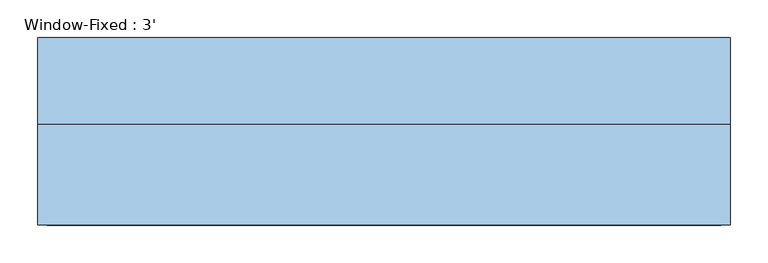
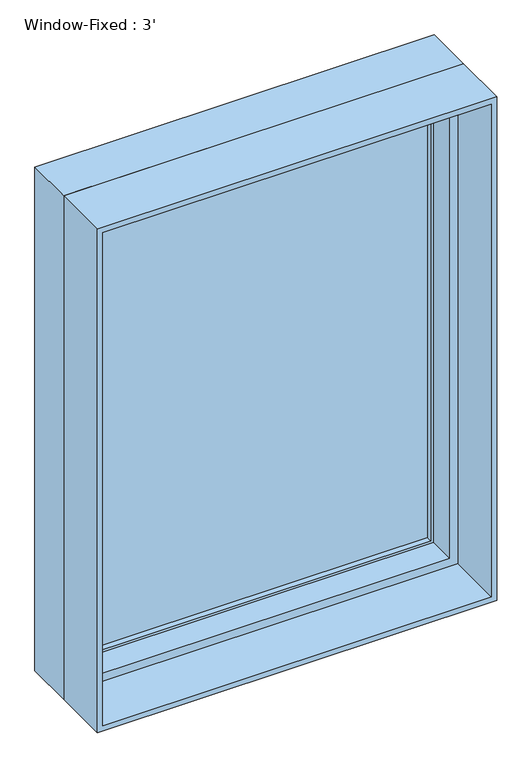
"""IFC4 building model written with IfcOpenShell, lengths in millimetres: window geometry, Window-Fixed : 3'."""

from ifc_helpers import new_model, si_unit, frame, origin, place, context, project, spatial, polyline, outline, extrude, faceted_brep, source, transform, mapped, element, save


def window_fixed_3_f41792bd(model_context):
    return source(origin(), model_context, "Body", "SolidModel", [
        faceted_brep([(457.2, 19.05, 2133.6), (457.2, 133.35, 2133.6), (-457.2, 133.35, 2133.6), (-457.2, 19.05, 2133.6), (-457.2, 133.35, 914.4), (-457.2, 19.05, 914.4), (457.2, 133.35, 914.4), (457.2, 19.05, 914.4), (425.45, 19.05, 2101.85), (425.45, 19.05, 946.15), (-425.45, 19.05, 946.15), (-425.45, 19.05, 2101.85), (-444.5, 133.35, 2120.9), (-444.5, 133.35, 927.1), (444.5, 133.35, 927.1), (444.5, 133.35, 2120.9), (425.45, 82.55, 2101.85), (-425.45, 82.55, 2101.85), (444.5, 82.55, 2120.9), (-444.5, 82.55, 2120.9), (-425.45, 82.55, 946.15), (-444.5, 82.55, 927.1), (425.45, 82.55, 946.15), (444.5, 82.55, 927.1)], [[[0, 1, 2, 3]], [[3, 2, 4, 5]], [[5, 4, 6, 7]], [[3, 5, 7, 0], [8, 9, 10, 11]], [[7, 6, 1, 0]], [[1, 6, 4, 2], [12, 13, 14, 15]], [[16, 8, 11, 17]], [[15, 18, 19, 12]], [[17, 11, 10, 20]], [[12, 19, 21, 13]], [[20, 10, 9, 22]], [[13, 21, 23, 14]], [[22, 9, 8, 16]], [[18, 23, 21, 19], [17, 20, 22, 16]], [[14, 23, 18, 15]]]),
        extrude(outline(polyline([(2133.6, -457.2), (914.4, -457.2), (914.4, 457.2), (2133.6, 457.2), (2133.6, -457.2)]), holes=[polyline([(2120.9, 444.5), (927.1, 444.5), (927.1, -444.5), (2120.9, -444.5), (2120.9, 444.5)])]), frame((0.0, -114.3, 0.0), z_axis=(0.0, 1.0, 0.0), x_axis=(0.0, 0.0, 1.0)), (0.0, 0.0, 1.0), 133.35),
        extrude(outline(polyline([(927.1, 444.5), (2120.9, 444.5), (2120.9, -444.5), (927.1, -444.5), (927.1, 444.5)]), holes=[polyline([(952.5, -419.1), (2095.5, -419.1), (2095.5, 419.1), (952.5, 419.1), (952.5, -419.1)])]), frame((0.0, 82.55, 0.0), z_axis=(0.0, 1.0, 0.0), x_axis=(0.0, 0.0, 1.0)), (0.0, 0.0, 1.0), 44.45),
        extrude(outline(polyline([(419.1, 114.3), (419.1, 107.95), (-419.1, 107.95), (-419.1, 114.3), (419.1, 114.3)])), frame((0.0, 0.0, 952.5), z_axis=(0.0, 0.0, 1.0), x_axis=(1.0, 0.0, 0.0)), (0.0, 0.0, 1.0), 1143.0),
        extrude(outline(polyline([(-419.1, 95.25), (-419.1, 101.6), (419.1, 101.6), (419.1, 95.25), (-419.1, 95.25)])), frame((0.0, 0.0, 952.5), z_axis=(0.0, 0.0, 1.0), x_axis=(1.0, 0.0, 0.0)), (0.0, 0.0, 1.0), 1143.0),
    ])


if __name__ == "__main__":
    model = new_model("IFC4")
    model_context = context("Model", 3, world=origin())
    ifc_project = project(units=[si_unit("LENGTHUNIT", "METRE", prefix="MILLI")], contexts=[model_context])
    site = spatial("IfcSite", under=ifc_project)
    building = spatial("IfcBuilding", under=site)
    placement = place(None, origin())
    window_fixed_3_shape = window_fixed_3_f41792bd(model_context)
    element("IfcWindow", 1, ObjectType="Window-Fixed : 3'", at=placement, inside=building, context=model_context, shape_type="MappedRepresentation", body=[
        mapped(window_fixed_3_shape, transform((0.0, 0.0, 0.0), x_axis=(1.0, 0.0, 0.0), y_axis=(0.0, 1.0, 0.0), z_axis=(0.0, 0.0, 1.0))),
    ])
    save(model, "model.ifc")

# Revit data of these elements
# Type "Window-Fixed : 3'"
#   Type Mark = "19"
#   Fire Rating = "0.5h"
#   Assembly Code = "B2020100"
#   Analytic Construction = "Double glazing - domestic"
#   Window Inset [instance default] = 0' - 0"
#   Wall Thickness [instance default] = 0' - 6"
#   Visual Light Transmittance = 0.81
#   Thermal Resistance (R) = 1.8146 (h·ft²·°F)/BTU
#   Solar Heat Gain Coefficient = 0.76
#   Rough Width = 3' - 0 1/2"
#   Rough Height = 4' - 0 1/2"
#   Interior Wall Closure [instance default] = 0' - 2 1/4"
#   Height = 4' - 0"
#   Heat Transfer Coefficient (U) = 0.5511 BTU/(h·ft²·°F)
#   Frame Extension [instance default] = 0' - 0 1/4"
#   Exterior Wall Closure [instance default] = 0' - 1 1/4"
#   Extension Jamb [instance default] = 0' - 2 1/4"
#   Default Sill Height = 3' - 0"
#   Width = 3' - 0"
#   Muntin Visibility = yes
#   Interior Trim Visibility [instance default] = yes
#   Exterior Trim Visibility [instance default] = yes
#   Extension Jamb Visibility [instance default] = yes
#   Muntin Pattern = Muntin Pattern_2x2 : Muntin Pattern_2x2
#   Interior Trim Material = Wood - Stained
#   Interior Trim = Trim-Window-Interior-Flat : Picture Frame
#   Interior Frame Material = Wood - Stained
#   Glass Panel Material = Glass
#   Exterior Trim Material = Clad - White
#   Exterior Trim = Trim-Window-Exterior-Flat : with Sill
#   Exterior Frame Material = Clad - White
#   Wall Closure = (empty or 0)
# Element 1 (IfcWindow, "Window-Fixed : 3'")
#   Wall Thickness = 0' - 9"
#   Extension Jamb = 0' - 5 1/4"
#   Materials on its faces: "Wood - Stained", "Glass", "Clad - White"
# Materials
#   "Wood - Stained": class "Wood", colour RGB 224 178 126, transparency 0, Cost = 0
#   "Glass": class "Glass", colour RGB 0 128 192, transparency 0.75, Description = "Soda Lime Glass", Cost = 0
#   "Clad - White": class "Wood", colour RGB 242 242 238, transparency 0, Cost = 0
